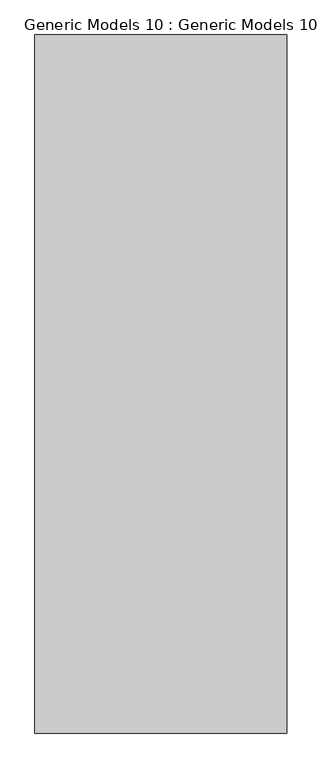
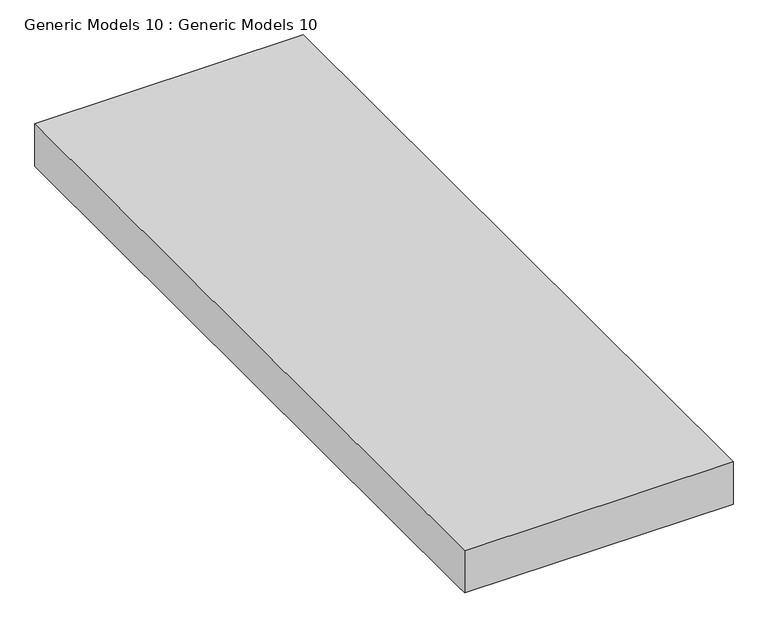
"""IFC4 building model written with IfcOpenShell, lengths in millimetres: proxy geometry, Generic Models 10 : Generic Models 10."""

from ifc_helpers import new_model, si_unit, frame, origin, place, context, project, spatial, polyline, outline, extrude, source, transform, mapped, element, save


def generic_models_10_generic_models_10_c1604470(model_context):
    return source(origin(), model_context, "Body", "SweptSolid", [
        extrude(outline(polyline([(9128.2444012, 2190.75), (9128.2444012, 2292.35), (10817.3444012, 2292.35), (10817.3444012, 2190.75), (10791.9444012, 2190.75), (9153.6444012, 2190.75), (9128.2444012, 2190.75)])), frame((-9091.7519453, 0.0, 0.0), z_axis=(1.0, 0.0, 0.0), x_axis=(0.0, 1.0, 0.0)), (0.0, 0.0, 1.0), 609.6),
    ])


if __name__ == "__main__":
    model = new_model("IFC4")
    model_context = context("Model", 3, world=origin())
    ifc_project = project(units=[si_unit("LENGTHUNIT", "METRE", prefix="MILLI")], contexts=[model_context])
    site = spatial("IfcSite", under=ifc_project)
    building = spatial("IfcBuilding", under=site)
    placement = place(None, origin())
    generic_models_10_generic_models_10_shape = generic_models_10_generic_models_10_c1604470(model_context)
    element("IfcBuildingElementProxy", 1, Name="Generic Models 10 : Generic Models 10", ObjectType="Generic Models 10 : Generic Models 10", at=placement, inside=building, context=model_context, shape_type="MappedRepresentation", body=[
        mapped(generic_models_10_generic_models_10_shape, transform((0.0, 0.0, 0.0), x_axis=(1.0, 0.0, 0.0), y_axis=(0.0, 1.0, 0.0), z_axis=(0.0, 0.0, 1.0))),
    ])
    save(model, "model.ifc")
